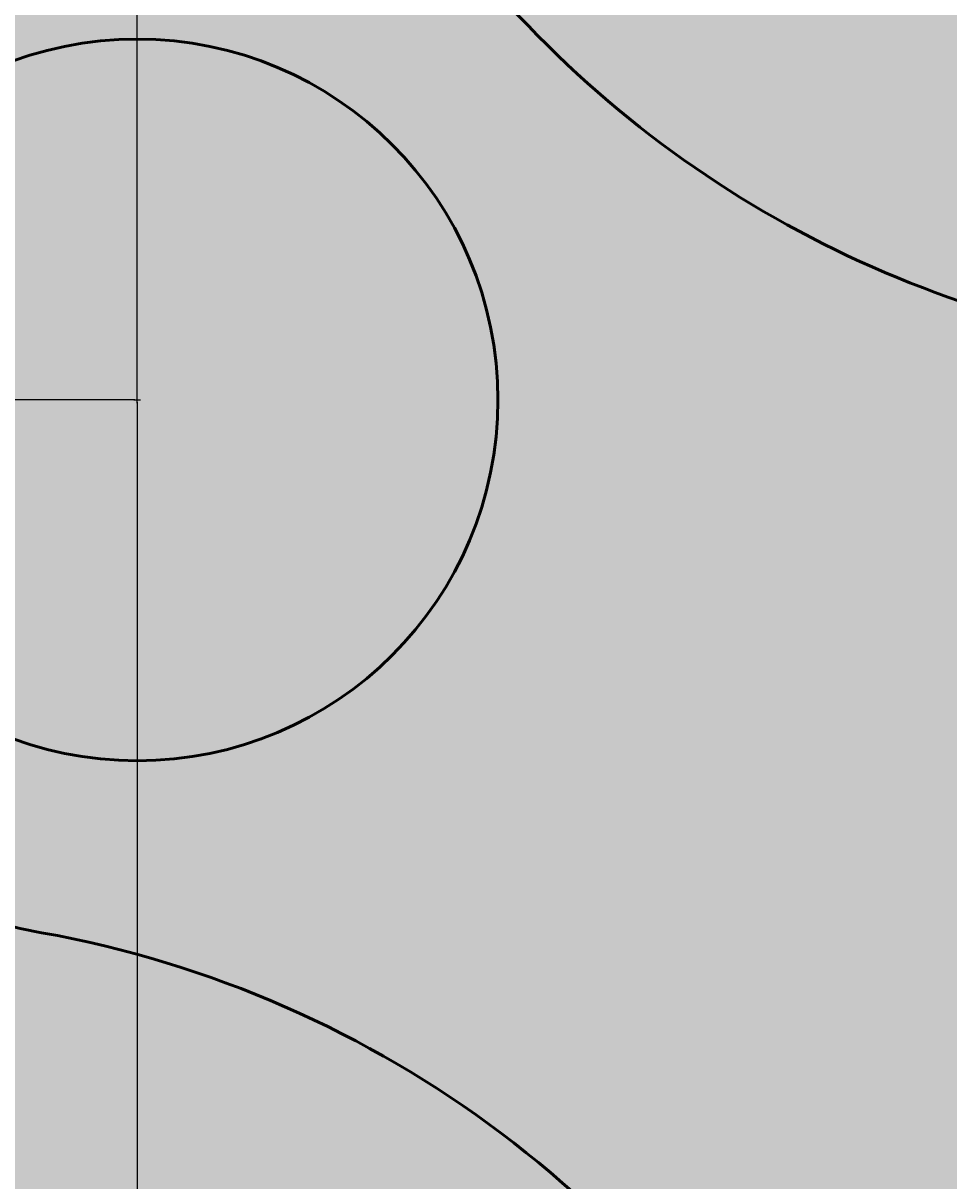
# Model space of a CAD drawing. Units: inches. Extents: x -31 to 87, y -18 to 100.
# Tile 4 of 7: x -8 to 18, y 52 to 84. Entities that reach past the tile are written whole.
import ezdxf

# ---------------------------------------------------------------- set-up
doc = ezdxf.new("R2010")
doc.units = ezdxf.units.IN
doc.header["$MEASUREMENT"] = 0
for name, color, linetype, lineweight in [('M-DIMS', 2, 'Continuous', 18), ('M-HATC', 7, 'Continuous', 18), ('M-OUTL', 4, 'Continuous', 50)]:
    doc.layers.add(name, color=color, linetype=linetype, lineweight=lineweight)
doc.styles.get("Standard").update_dxf_attribs({"font": 'arial.ttf'})
doc.dimstyles.get("Standard").update_dxf_attribs({"dimtxt": 0.18, "dimasz": 0.18, "dimexe": 0.18, "dimexo": 0.0625, "dimgap": 0.09, "dimtad": 0, "dimtih": 1, "dimtoh": 1, "dimdec": 4, "dimzin": 0, "dimdsep": 46, "dimtxsty": 'Standard', "dimcen": 0.09, "dimadec": 0, "dimazin": 0, "dimtfac": 1, "dimtdec": 4, "dimtofl": 0, "dimtmove": 0, "dimatfit": 3, "dimfxl": 1, "dimtolj": 1, "dimtzin": 0, "dimarcsym": 0})

# ---------------------------------------------------------------- blocks, each defined once
blk = doc.blocks.new('*D1')
at = {"layer": 'Defpoints', "color": 0, "transparency": 16777216}
for p in [(-24.622, 75.027), (80.28, 72.235), (80.28, -17.851)]:
    blk.add_point(p, dxfattribs=at)
at = {"layer": 'M-DIMS', "color": 0, "lineweight": -2, "transparency": 16777216}
for p, q in [((-24.622, 74.965), (-24.622, -18.031)), ((80.28, 72.173), (80.28, -18.031)), ((-24.442, -17.851), (27.443, -17.851)), ((80.1, -17.851), (28.214, -17.851))]:
    blk.add_line(p, q, dxfattribs=at)
at = {"layer": 'M-DIMS', "color": 0, "transparency": 16777216}
for points in [[(-24.442, -17.821), (-24.442, -17.881), (-24.622, -17.851)], [(80.1, -17.821), (80.1, -17.881), (80.28, -17.851)]]:
    blk.add_solid(points, dxfattribs=at)
at = {"layer": 'M-DIMS', "color": 0, "transparency": 16777216, "insert": (27.829, -17.851), "char_height": 0.18, "attachment_point": 5}
blk.add_mtext('\\A1;104.9', dxfattribs=at)
blk = doc.blocks.new('*D3')
at = {"layer": 'Defpoints', "color": 0, "transparency": 16777216}
for p in [(60.319, 99.89), (-4.681, 73.49), (60.319, 73.49)]:
    blk.add_point(p, dxfattribs=at)
at = {"layer": 'M-DIMS', "color": 0, "lineweight": -2, "transparency": 16777216}
for p, q in [((-4.681, 73.552), (-4.681, 100.07)), ((-4.501, 99.89), (27.599, 99.89)), ((60.139, 99.89), (28.039, 99.89)), ((60.319, 73.552), (60.319, 100.07))]:
    blk.add_line(p, q, dxfattribs=at)
at = {"layer": 'M-DIMS', "color": 0, "transparency": 16777216}
for points in [[(-4.501, 99.92), (-4.501, 99.86), (-4.681, 99.89)], [(60.139, 99.92), (60.139, 99.86), (60.319, 99.89)]]:
    blk.add_solid(points, dxfattribs=at)
at = {"layer": 'M-DIMS', "color": 0, "transparency": 16777216, "insert": (27.819, 99.89), "char_height": 0.18, "attachment_point": 5}
blk.add_mtext('\\A1;65', dxfattribs=at)
blk = doc.blocks.new('*D4')
at = {"layer": 'Defpoints', "color": 0, "transparency": 16777216}
for p in [(-4.681, 73.49), (27.319, 8.49), (27.319, -17.851)]:
    blk.add_point(p, dxfattribs=at)
at = {"layer": 'M-DIMS', "color": 0, "lineweight": -2, "transparency": 16777216}
for p, q in [((-4.681, 73.427), (-4.681, -18.031)), ((27.319, 8.427), (27.319, -18.031)), ((-4.501, -17.851), (11.101, -17.851)), ((27.139, -17.851), (11.537, -17.851))]:
    blk.add_line(p, q, dxfattribs=at)
at = {"layer": 'M-DIMS', "color": 0, "transparency": 16777216}
for points in [[(-4.501, -17.821), (-4.501, -17.881), (-4.681, -17.851)], [(27.139, -17.821), (27.139, -17.881), (27.319, -17.851)]]:
    blk.add_solid(points, dxfattribs=at)
at = {"layer": 'M-DIMS', "color": 0, "transparency": 16777216, "insert": (11.319, -17.851), "char_height": 0.18, "attachment_point": 5}
blk.add_mtext('\\A1;32', dxfattribs=at)
blk = doc.blocks.new('*D5')
at = {"layer": 'Defpoints', "color": 0, "transparency": 16777216}
for p in [(-31.022, 73.49), (-4.681, 73.49), (27.319, 8.49)]:
    blk.add_point(p, dxfattribs=at)
at = {"layer": 'M-DIMS', "color": 0, "lineweight": -2, "transparency": 16777216}
for p, q in [((-4.744, 73.49), (-31.202, 73.49)), ((-31.022, 73.31), (-31.022, 41.172)), ((-31.022, 8.67), (-31.022, 40.808)), ((27.256, 8.49), (-31.202, 8.49))]:
    blk.add_line(p, q, dxfattribs=at)
at = {"layer": 'M-DIMS', "color": 0, "transparency": 16777216}
for points in [[(-31.052, 73.31), (-30.992, 73.31), (-31.022, 73.49)], [(-31.052, 8.67), (-30.992, 8.67), (-31.022, 8.49)]]:
    blk.add_solid(points, dxfattribs=at)
at = {"layer": 'M-DIMS', "color": 0, "transparency": 16777216, "insert": (-31.022, 40.99), "char_height": 0.18, "attachment_point": 5}
blk.add_mtext('\\A1;65', dxfattribs=at)
blk = doc.blocks.new('*D8')
at = {"layer": 'Defpoints', "color": 0, "transparency": 16777216}
for p in [(4.958, 84.983), (-4.681, 73.49)]:
    blk.add_point(p, dxfattribs=at)
at = {"layer": 'M-DIMS', "color": 0, "lineweight": -2, "transparency": 16777216}
for p, q in [((10.741, 91.879), (5.073, 85.121)), ((10.921, 91.879), (10.741, 91.879)), ((-4.771, 73.49), (-4.591, 73.49)), ((-4.681, 73.4), (-4.681, 73.58))]:
    blk.add_line(p, q, dxfattribs=at)
at = {"layer": 'M-DIMS', "color": 0, "transparency": 16777216}
blk.add_solid([(5.05, 85.14), (5.096, 85.102), (4.958, 84.983)], dxfattribs=at)
at = {"layer": 'M-DIMS', "color": 0, "transparency": 16777216, "insert": (11.42, 91.879), "char_height": 0.18, "attachment_point": 5}
blk.add_mtext('\\A1;3X R15', dxfattribs=at)

msp = doc.modelspace()

# ---------------------------------------------------------------- hatches: boundary and pattern name
at = {"layer": 'M-HATC'}
h = msp.add_hatch(color=256, dxfattribs=at)
h.set_gradient(color1=(205, 32, 39), color2=(247, 242, 129))
h.paths.add_polyline_path([(-2.425, 93.362, 0.593504), (-22.614, 64.635), (8.64, 1.342, 0.746388), (46.874, 4.293), (79.436, 67.614, 0.505151), (60.278, 93.49)])
h.paths.add_polyline_path([(49.486, 83.865, -1.392259), (62.663, 58.674, 0.510547), (40.663, 15.341, -1.641082), (14.002, 15.393, 0.505248), (-7.332, 58.726, -1.377138), (6.152, 83.865, 0.426931)], flags=16)
h.paths.add_polyline_path([(5.319, 73.49, -1), (-14.681, 73.49, -1)], flags=0)
h.paths.add_polyline_path([(70.319, 73.49, -1), (50.319, 73.49, -1)], flags=0)
h.paths.add_polyline_path([(37.319, 8.49, -1), (17.319, 8.49, -1)], flags=0)
h.paths.add_polyline_path([(6.152, 83.865, 1.377138), (-7.332, 58.726, -0.505248), (14.002, 15.393, 1.641082), (40.663, 15.341, -0.510547), (62.663, 58.674, 1.392259), (49.486, 83.865, -0.426931)], flags=0)
h = msp.add_hatch(color=256, dxfattribs=at)
h.dxf.hatch_style = 1
h.paths.add_polyline_path([(5.319, 73.49, 1), (-14.681, 73.49, 1)])
h.paths.add_polyline_path([(50.319, 73.49, 1), (70.319, 73.49, 1)])
h.paths.add_polyline_path([(37.319, 8.49, 1), (17.319, 8.49, 1)])

# ---------------------------------------------------------------- linework, layer by layer
at = {"layer": 'M-OUTL'}
msp.add_circle((-4.681, 73.49), 10, dxfattribs=at)
for centre, radius, start, end in [((-4.681, 73.49), 20, 83.5229, 206.2801), ((-4.681, 73.49), 15, 43.7617, 259.8216), ((27.819, 104.615), 30, 223.7617, 316.2383), ((-12.633, 29.198), 30, 332.6011, 79.8216)]:
    msp.add_arc(centre, radius, start, end, dxfattribs=at)

# ---------------------------------------------------------------- dimensions: what is measured, and where the dimension line sits
at = {"layer": 'M-DIMS'}
for base, p1, p2, override, picture, middle in [((60.319, 99.89), (-4.681, 73.49), (60.319, 73.49), {"dimdec": 0, "dimlfac": 1, "dimrnd": 0, "dimzin": 0, "dimdsep": 46, "dimlunit": 2}, '*D3', (27.819, 99.89)), ((80.28, -17.851), (-24.622, 75.027), (80.28, 72.235), {"dimdec": 1, "dimlfac": 1, "dimrnd": 0, "dimzin": 0, "dimdsep": 46, "dimlunit": 2}, '*D1', (27.829, -17.851)), ((27.319, -17.851), (-4.681, 73.49), (27.319, 8.49), {"dimdec": 0, "dimlfac": 1, "dimrnd": 0, "dimzin": 0, "dimdsep": 46, "dimlunit": 2}, '*D4', (11.319, -17.851))]:
    dim = msp.add_linear_dim(base=base, p1=p1, p2=p2, dimstyle='Standard', override=override, dxfattribs=at)
    dim.commit()
    dim.dimension.update_dxf_attribs({"geometry": picture, "text_midpoint": middle})
dim = msp.add_radius_dim(center=(-4.681, 73.49), mpoint=(4.958, 84.983), text='3X <>', dimstyle='Standard', override={"dimdec": 0, "dimlfac": 1, "dimrnd": 0, "dimzin": 0, "dimdsep": 46, "dimlunit": 2}, dxfattribs=at)
dim.commit()
dim.dimension.update_dxf_attribs({"geometry": '*D8', "text_midpoint": (11.42, 91.879), "dimtype": 164})
dim = msp.add_linear_dim(base=(-31.022, 73.49), p1=(27.319, 8.49), p2=(-4.681, 73.49), angle=90, dimstyle='Standard', override={"dimdec": 0, "dimlfac": 1, "dimrnd": 0, "dimzin": 0, "dimdsep": 46, "dimlunit": 2}, dxfattribs=at)
dim.commit()
dim.dimension.update_dxf_attribs({"geometry": '*D5', "text_midpoint": (-31.022, 40.99)})

doc.saveas('drawing.dxf')
